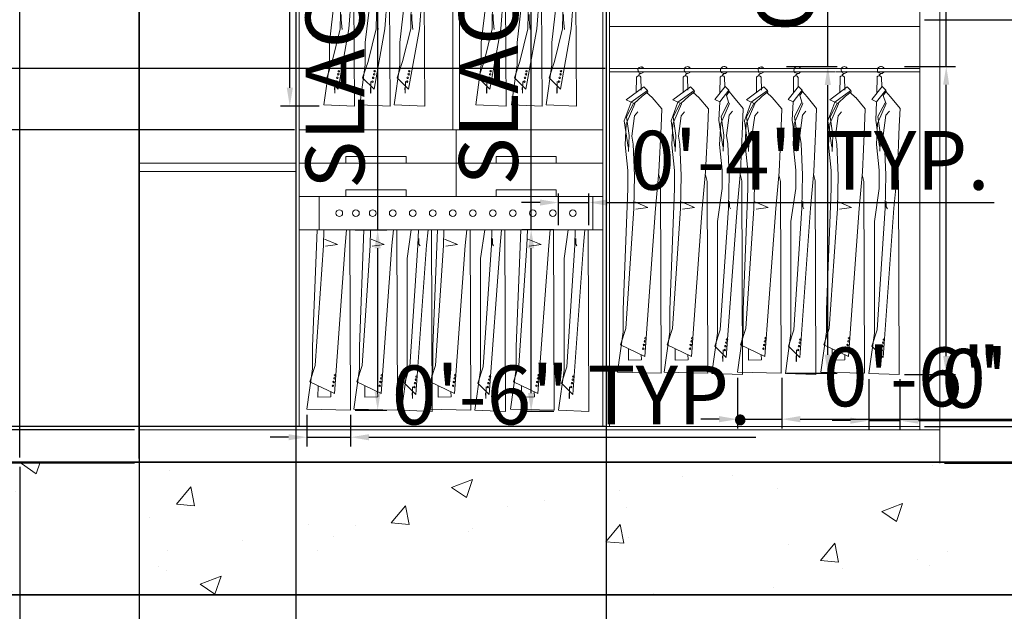
# Model space of a CAD drawing. Units: inches. Extents: x 2257 to 3678, y 834 to 1975.
# Tile 12 of 16: x 3338 to 3471, y 1677 to 1757. Entities that reach past the tile are written whole.
import ezdxf

# ---------------------------------------------------------------- set-up
doc = ezdxf.new("R2010")
doc.units = ezdxf.units.IN
for name, color, linetype, lineweight in [('A-ANNO-DIMS', 2, 'Continuous', 18), ('A-FURN-ELEV', 8, 'Continuous', 13), ('A-SECT', 7, 'Continuous', 35), ('A-SECT-CONC-PATT', 252, 'Continuous', 13)]:
    doc.layers.add(name, color=color, linetype=linetype, lineweight=lineweight)
doc.styles.get("Standard").update_dxf_attribs({"font": 'arial.ttf'})
doc.dimstyles.new('ISO-25', dxfattribs={"dimtxt": 8, "dimasz": 2.5, "dimexe": 1.25, "dimexo": 0.625, "dimtad": 1, "dimdec": 0, "dimlunit": 3, "dimtxsty": 'Standard', "dimcen": 2.5, "dimadec": 0, "dimazin": 0, "dimtfac": 1, "dimtdec": 0, "dimtmove": 0, "dimatfit": 3, "dimfxl": 1, "dimarcsym": 0})

# ---------------------------------------------------------------- blocks, each defined once
blk = doc.blocks.new('WARDROBE-JACKET-SHORT')
for p, q in [((1.8, 28.09), (0.39, 26.33)), ((1.11, 29.37), (1.09, 27.21)), ((1.75, 28.02), (1.71, 29.34)), ((1.8, 28.09), (2.29, 27.6)), ((1.06, 26.01), (2.29, 27.6)), ((2.34, 27.43), (1.96, 26.84)), ((2.29, 25.81), (1.96, 26.84)), ((2.34, 27.43), (2.29, 27.6)), ((2.33, 27.41), (2.93, 26.66)), ((0.39, 26.33), (1.06, 26.01)), ((1.06, 26.01), (0.94, 23.49)), ((2.36, 25.78), (1.19, 23.07)), ((1.23, 24.01), (2.2, 25.86)), ((2.94, 26.66), (4.23, 25.09)), ((1.96, 21.41), (2.32, 24.17)), ((2.32, 24.17), (2.79, 24.73)), ((4.23, 25.09), (4.14, 22.7)), ((0.94, 23.49), (1.46, 19.92)), ((1.19, 23.07), (1.04, 20.22)), ((1.23, 24.01), (1.59, 21.47)), ((1.59, 21.47), (1.5, 19.31)), ((2.14, 20.31), (1.96, 21.41)), ((4.14, 22.7), (3.87, 16.54)), ((1.04, 20.22), (1.4, 16.72)), ((2.32, 16.07), (2.14, 20.31)), ((1.4, 16.72), (1.4, 14.23)), ((2.23, 10.49), (2.32, 16.07)), ((3.87, 16.54), (3.41, 10.49)), ((4.05, 15.25), (3.83, 16.16)), ((4.14, 0), (4.05, 15.25)), ((1.4, 14.23), (0.76, 8.65)), ((2.37, 12.45), (2.37, 11.72)), ((2.37, 11.72), (2.51, 10.41)), ((1.13, 6.07), (2.23, 10.49)), ((3.41, 10.49), (1.94, 2.29)), ((0.76, 8.65), (0.76, 5.61)), ((0.76, 5.61), (0, 0.16)), ((0.4, 3.86), (1.13, 6.07)), ((1.94, 2.29), (0.4, 3.86)), ((1.51, 3.33), (1.49, 1.77)), ((1.47, 1.8), (1.45, 2.53)), ((1.49, 1.77), (1.47, 1.8)), ((0, 0.16), (4.14, 0))]:
    blk.add_line(p, q)
for centre, radius in [((1.45, 30.04), 0.0434), ((1.96, 4.32), 0.103), ((2.03, 4.74), 0.103), ((1.74, 3.32), 0.103), ((1.83, 3.84), 0.103)]:
    blk.add_circle(centre, radius)
for centre, radius, start, end in [((1.64, 30.31), 0.481, 28.9305, 230.329), ((1.4, 29.2), 0.341, 24.2419, 150.7783), ((1.75, 29.53), 0.361, 98.1438, 177.8717), ((1.75, 29.53), 0.315, 98.1438, 177.7449), ((1.64, 30.31), 0.481, 278.1438, 332.6972)]:
    blk.add_arc(centre, radius, start, end)
blk = doc.blocks.new('WARDROBE-JACKET-SHORT-B')
for p, q in [((1.11, 29.37), (1.09, 27.21)), ((1.75, 28.02), (1.72, 29.34)), ((1.8, 28.09), (2.29, 27.6)), ((1.06, 26.01), (2.29, 27.6)), ((2.34, 27.43), (1.96, 26.84)), ((2.29, 25.81), (1.96, 26.84)), ((2.34, 27.43), (2.29, 27.6)), ((2.33, 27.41), (2.94, 26.66)), ((1.06, 26.01), (0.94, 23.49)), ((2.36, 25.78), (1.19, 23.07)), ((1.23, 24.01), (2.2, 25.86)), ((2.94, 26.66), (4.23, 25.09)), ((1.96, 21.41), (2.33, 24.17)), ((2.33, 24.17), (2.79, 24.73)), ((4.23, 25.09), (4.14, 22.7)), ((0.94, 23.49), (1.46, 19.92)), ((1.19, 23.07), (1.04, 20.22)), ((1.23, 24.01), (1.59, 21.47)), ((1.59, 21.47), (1.5, 19.31)), ((2.14, 20.31), (1.96, 21.41)), ((4.14, 22.7), (3.87, 16.54)), ((1.04, 20.22), (1.4, 16.72)), ((2.33, 16.07), (2.14, 20.31)), ((1.4, 16.72), (1.4, 14.23)), ((2.23, 10.49), (2.33, 16.07)), ((3.87, 16.54), (3.41, 10.49)), ((4.05, 15.25), (3.83, 16.16)), ((4.14, 0), (4.05, 15.25)), ((1.4, 14.23), (0.76, 8.65)), ((2.37, 12.45), (2.37, 11.72)), ((2.37, 11.72), (2.52, 10.41)), ((1.13, 6.07), (2.23, 10.49)), ((3.41, 10.49), (1.94, 2.29)), ((0.76, 8.65), (0.76, 5.61)), ((0.76, 5.61), (0, 0.16)), ((0.4, 3.86), (1.13, 6.07)), ((1.94, 2.29), (0.4, 3.86)), ((1.51, 3.33), (1.49, 1.77)), ((1.47, 1.8), (1.45, 2.53)), ((1.49, 1.77), (1.47, 1.8)), ((0, 0.16), (4.14, 0))]:
    blk.add_line(p, q)
for centre, radius in [((1.45, 30.04), 0.0434), ((1.96, 4.32), 0.103), ((2.03, 4.74), 0.103), ((1.74, 3.32), 0.103), ((1.83, 3.84), 0.103)]:
    blk.add_circle(centre, radius)
for centre, radius, start, end in [((1.4, 29.2), 0.341, 24.2419, 150.7783), ((1.67, 30.37), 0.367, 58.8889, 230.4094), ((1.75, 29.53), 0.361, 98.1438, 177.8717), ((1.75, 29.53), 0.315, 98.1438, 177.7449), ((1.64, 30.31), 0.481, 278.1438, 332.6972), ((1.64, 30.31), 0.481, 28.9305, 58.8889)]:
    blk.add_arc(centre, radius, start, end)
blk = doc.blocks.new('WARDROBE-COAT')
for p, q in [((2.59, 40.24), (2.57, 38.08)), ((3.24, 38.47), (3.19, 40.21)), ((3.58, 38.9), (1.2, 37.14)), ((3.58, 38.9), (4.07, 38.41)), ((1.87, 36.82), (4.07, 38.41)), ((2.29, 36.62), (3.34, 37.65)), ((4.11, 38.23), (3.34, 37.65)), ((3.96, 38.12), (4.71, 37.47)), ((4.11, 38.23), (4.07, 38.41)), ((4.72, 37.47), (6.01, 35.9)), ((1.87, 36.82), (0.94, 34.3)), ((2.36, 36.59), (1.19, 33.88)), ((1.2, 37.14), (2.36, 36.59)), ((1.23, 34.82), (2.2, 36.66)), ((1.23, 34.82), (1.59, 32.28)), ((1.96, 32.22), (2.33, 34.98)), ((2.33, 34.98), (2.79, 35.53)), ((6.01, 35.9), (5.92, 33.51)), ((0.94, 34.3), (1.46, 30.72)), ((1.19, 33.88), (1.04, 31.02)), ((5.92, 33.51), (5.64, 27.34)), ((1.59, 32.28), (1.5, 30.12)), ((2.14, 31.12), (1.96, 32.22)), ((1.04, 31.02), (1.4, 27.53)), ((2.33, 26.88), (2.14, 31.12)), ((1.4, 27.53), (1.4, 25.04)), ((2.23, 22.37), (2.33, 26.88)), ((5.64, 27.34), (5.18, 22.37)), ((5.83, 26.06), (5.61, 26.97)), ((5.92, 0), (5.83, 26.06)), ((1.4, 25.04), (0.76, 8.65)), ((2.37, 23.26), (4.14, 22.52)), ((1.13, 6.07), (2.23, 22.37)), ((4.14, 22.52), (2.52, 22.29)), ((5.18, 22.37), (3.72, 2.29)), ((0.76, 8.65), (0.76, 5.61)), ((0.76, 5.61), (0, 0.16)), ((0.4, 3.86), (1.13, 6.07)), ((3.72, 2.29), (0.4, 3.86)), ((1.51, 3.33), (1.49, 1.77)), ((1.49, 1.77), (3.25, 1.8)), ((3.25, 1.8), (3.22, 2.53)), ((0, 0.16), (5.92, 0))]:
    blk.add_line(p, q)
for centre, radius in [((2.93, 40.91), 0.0434), ((3.74, 4.32), 0.103), ((3.81, 4.74), 0.103), ((3.52, 3.32), 0.103), ((3.61, 3.84), 0.103)]:
    blk.add_circle(centre, radius)
for centre, radius, start, end in [((3.15, 41.24), 0.367, 58.8889, 230.4094), ((3.12, 41.19), 0.481, 28.9305, 58.8889), ((2.88, 40.07), 0.341, 24.2419, 150.7783), ((3.23, 40.4), 0.361, 98.1438, 177.8717), ((3.23, 40.4), 0.315, 98.1438, 177.7449), ((3.12, 41.19), 0.481, 278.1438, 332.6972)]:
    blk.add_arc(centre, radius, start, end)
blk = doc.blocks.new('WARDROBE-COAT-B')
for p, q in [((2.59, 40.24), (2.57, 38.08)), ((3.24, 38.47), (3.19, 40.21)), ((3.58, 38.9), (1.2, 37.14)), ((3.58, 38.9), (4.07, 38.41)), ((1.87, 36.82), (4.07, 38.41)), ((2.29, 36.62), (3.34, 37.65)), ((4.11, 38.23), (3.34, 37.65)), ((3.96, 38.12), (4.71, 37.47)), ((4.11, 38.23), (4.07, 38.41)), ((4.72, 37.47), (6.01, 35.9)), ((1.87, 36.82), (0.94, 34.3)), ((2.36, 36.59), (1.19, 33.88)), ((1.2, 37.14), (2.36, 36.59)), ((1.23, 34.82), (2.2, 36.66)), ((1.23, 34.82), (1.59, 32.28)), ((1.96, 32.22), (2.33, 34.98)), ((2.33, 34.98), (2.79, 35.53)), ((6.01, 35.9), (5.92, 33.51)), ((0.94, 34.3), (1.46, 30.72)), ((1.19, 33.88), (1.04, 31.02)), ((5.92, 33.51), (5.64, 27.34)), ((1.59, 32.28), (1.5, 30.12)), ((2.14, 31.12), (1.96, 32.22)), ((1.04, 31.02), (1.4, 27.53)), ((2.33, 26.88), (2.14, 31.12)), ((1.4, 27.53), (1.4, 25.04)), ((2.23, 22.37), (2.33, 26.88)), ((5.64, 27.34), (5.18, 22.37)), ((5.83, 26.06), (5.61, 26.97)), ((5.92, 0), (5.83, 26.06)), ((1.4, 25.04), (0.76, 8.65)), ((2.37, 23.26), (4.14, 22.52)), ((1.13, 6.07), (2.23, 22.37)), ((4.14, 22.52), (2.52, 22.29)), ((5.18, 22.37), (3.72, 2.29)), ((0.76, 8.65), (0.76, 5.61)), ((0.76, 5.61), (0, 0.16)), ((0.4, 3.86), (1.13, 6.07)), ((3.72, 2.29), (0.4, 3.86)), ((1.51, 3.33), (1.49, 1.77)), ((1.49, 1.77), (3.25, 1.8)), ((3.25, 1.8), (3.22, 2.53)), ((0, 0.16), (5.92, 0))]:
    blk.add_line(p, q)
for centre, radius in [((2.93, 40.91), 0.0434), ((3.74, 4.32), 0.103), ((3.81, 4.74), 0.103), ((3.52, 3.32), 0.103), ((3.61, 3.84), 0.103)]:
    blk.add_circle(centre, radius)
for centre, radius, start, end in [((3.15, 41.24), 0.412, 58.8889, 230.4094), ((3.12, 41.19), 0.481, 28.9305, 58.8889), ((2.88, 40.07), 0.341, 24.2419, 150.7783), ((3.23, 40.4), 0.361, 98.1438, 177.8717), ((3.23, 40.4), 0.315, 98.1438, 177.7449), ((3.12, 41.19), 0.481, 278.1438, 332.6972)]:
    blk.add_arc(centre, radius, start, end)
blk = doc.blocks.new('WARDROBE-JACKET-LONG')
for p, q in [((1.11, 40.4), (1.09, 38.25)), ((1.75, 39.06), (1.72, 40.38)), ((1.8, 39.13), (0.39, 37.37)), ((1.8, 39.13), (2.29, 38.64)), ((1.06, 37.05), (2.29, 38.64)), ((2.34, 38.46), (1.96, 37.88)), ((2.29, 36.85), (1.96, 37.88)), ((2.34, 38.46), (2.29, 38.64)), ((2.33, 38.45), (2.94, 37.7)), ((2.94, 37.7), (4.24, 36.13)), ((0.39, 37.37), (1.06, 37.05)), ((1.06, 37.05), (0.94, 34.53)), ((2.36, 36.82), (1.19, 34.11)), ((1.23, 35.05), (2.2, 36.89)), ((4.24, 36.13), (4.14, 33.74)), ((1.23, 35.05), (1.59, 32.51)), ((1.96, 32.45), (2.33, 35.21)), ((2.33, 35.21), (2.79, 35.76)), ((0.94, 34.53), (1.46, 30.95)), ((1.19, 34.11), (1.04, 31.25)), ((4.14, 33.74), (3.87, 27.57)), ((1.59, 32.51), (1.5, 30.35)), ((2.14, 31.35), (1.96, 32.45)), ((1.04, 31.25), (1.4, 27.76)), ((2.33, 27.11), (2.14, 31.35)), ((1.4, 27.76), (1.4, 25.27)), ((2.23, 22.6), (2.33, 27.11)), ((3.87, 27.57), (3.41, 22.6)), ((4.05, 26.29), (3.83, 27.2)), ((4.14, 0), (4.05, 26.29)), ((1.4, 25.27), (0.76, 20.76)), ((2.37, 23.49), (2.37, 22.75)), ((2.37, 22.75), (2.52, 22.52)), ((1.13, 6.07), (2.23, 22.6)), ((3.41, 22.6), (1.94, 2.29)), ((0.76, 20.76), (0.76, 5.61)), ((0.76, 5.61), (0, 0.15)), ((0.4, 3.86), (1.13, 6.07)), ((1.94, 2.29), (0.4, 3.86)), ((1.51, 3.33), (1.49, 1.77)), ((1.47, 1.8), (1.45, 2.52)), ((1.49, 1.77), (1.47, 1.8)), ((0, 0.15), (4.14, 0))]:
    blk.add_line(p, q)
for centre, radius in [((1.45, 41.08), 0.0434), ((1.96, 4.32), 0.103), ((2.03, 4.74), 0.103), ((1.74, 3.32), 0.103), ((1.83, 3.84), 0.103)]:
    blk.add_circle(centre, radius)
for centre, radius, start, end in [((1.64, 41.35), 0.481, 28.9305, 230.329), ((1.4, 40.24), 0.341, 24.2419, 150.7783), ((1.75, 40.56), 0.361, 98.1438, 177.8717), ((1.75, 40.56), 0.315, 98.1438, 177.7449), ((1.64, 41.35), 0.481, 278.1438, 332.6972)]:
    blk.add_arc(centre, radius, start, end)
blk = doc.blocks.new('WARDROBE-GARMENT-LOWER')
for p, q in [((1.38, 24.51), (0.76, 8.65)), ((2.23, 22.37), (2.28, 24.51)), ((5.38, 24.51), (5.18, 22.37)), ((5.92, 0), (5.83, 24.51)), ((2.37, 23.26), (4.14, 22.52)), ((1.13, 6.07), (2.23, 22.37)), ((4.14, 22.52), (2.52, 22.29)), ((5.18, 22.37), (3.72, 2.29)), ((0.76, 8.65), (0.76, 5.61)), ((0.76, 5.61), (0, 0.16)), ((0.4, 3.86), (1.13, 6.07)), ((3.72, 2.29), (0.4, 3.86)), ((1.51, 3.33), (1.49, 1.77)), ((1.49, 1.77), (3.25, 1.8)), ((3.25, 1.8), (3.22, 2.52)), ((0, 0.16), (5.92, 0))]:
    blk.add_line(p, q)
for centre in [(3.74, 4.32), (3.81, 4.74), (3.52, 3.32), (3.61, 3.84)]:
    blk.add_circle(centre, 0.103)
blk = doc.blocks.new('WARDROBE-GARMENT-LOWER-B')
for p, q in [((1.32, 24.68), (0.76, 20.76)), ((2.23, 22.6), (2.28, 24.68)), ((3.6, 24.68), (3.41, 22.6)), ((4.14, 0), (4.06, 24.68)), ((2.37, 23.49), (2.37, 22.75)), ((2.37, 22.75), (2.51, 22.52)), ((1.13, 6.07), (2.23, 22.6)), ((3.41, 22.6), (1.94, 2.29)), ((0.76, 20.76), (0.76, 5.61)), ((0.76, 5.61), (0, 0.16)), ((0.4, 3.86), (1.13, 6.07)), ((1.94, 2.29), (0.4, 3.86)), ((1.51, 3.33), (1.49, 1.77)), ((1.47, 1.8), (1.45, 2.53)), ((1.49, 1.77), (1.47, 1.8)), ((0, 0.16), (4.14, 0))]:
    blk.add_line(p, q)
for centre in [(1.96, 4.32), (2.03, 4.74), (1.74, 3.32), (1.83, 3.84)]:
    blk.add_circle(centre, 0.103)
blk = doc.blocks.new('*D86')
at = {"layer": 'A-ANNO-DIMS', "color": 0, "lineweight": -2, "transparency": 16777216}
for p, q in [((3374.38, 1776.04), (3374.38, 1916.69)), ((3378.38, 1776.04), (3373.13, 1776.04)), ((3374.38, 1747.73), (3374.38, 1773.54)), ((3378.38, 1745.23), (3373.13, 1745.23))]:
    blk.add_line(p, q, dxfattribs=at)
at = {"layer": 'A-ANNO-DIMS', "color": 0, "transparency": 16777216}
for points in [[(3373.96, 1773.54), (3374.8, 1773.54), (3374.38, 1776.04)], [(3373.96, 1747.73), (3374.8, 1747.73), (3374.38, 1745.23)]]:
    blk.add_solid(points, dxfattribs=at)
at = {"layer": 'Defpoints', "color": 0, "transparency": 16777216}
for p in [(3374.38, 1776.04), (3379, 1776.04), (3379, 1745.23)]:
    blk.add_point(p, dxfattribs=at)
at = {"layer": 'A-ANNO-DIMS', "color": 0, "transparency": 16777216, "insert": (3369.62, 1847.62), "char_height": 8, "attachment_point": 5, "rotation": 90}
blk.add_mtext('SHORT JACKET 2\'-7" TYP.', dxfattribs=at)
blk = doc.blocks.new('*D88')
at = {"layer": 'A-ANNO-DIMS', "color": 0, "lineweight": -2, "transparency": 16777216}
for p, q in [((3386.31, 1728.42), (3386.31, 1846.75)), ((3383.26, 1728.42), (3387.56, 1728.42)), ((3386.31, 1706.41), (3386.31, 1725.92)), ((3383.26, 1703.91), (3387.56, 1703.91))]:
    blk.add_line(p, q, dxfattribs=at)
at = {"layer": 'A-ANNO-DIMS', "color": 0, "transparency": 16777216}
for points in [[(3385.89, 1725.92), (3386.72, 1725.92), (3386.31, 1728.42)], [(3385.89, 1706.41), (3386.72, 1706.41), (3386.31, 1703.91)]]:
    blk.add_solid(points, dxfattribs=at)
at = {"layer": 'Defpoints', "color": 0, "transparency": 16777216}
for p in [(3382.63, 1728.42), (3386.31, 1728.42), (3382.63, 1703.91)]:
    blk.add_point(p, dxfattribs=at)
at = {"layer": 'A-ANNO-DIMS', "color": 0, "transparency": 16777216, "insert": (3381.55, 1788.84), "char_height": 8, "attachment_point": 5, "rotation": 90}
blk.add_mtext('SLACKS 2\'-0 1/2" TYP.', dxfattribs=at)
blk = doc.blocks.new('*D89')
at = {"layer": 'A-ANNO-DIMS', "color": 0, "lineweight": -2, "transparency": 16777216}
for p, q in [((3376.71, 1703.29), (3376.71, 1698.99)), ((3382.63, 1703.29), (3382.63, 1698.99)), ((3374.21, 1700.24), (3371.71, 1700.24)), ((3376.71, 1700.24), (3382.63, 1700.24)), ((3385.13, 1700.24), (3437.65, 1700.24))]:
    blk.add_line(p, q, dxfattribs=at)
at = {"layer": 'A-ANNO-DIMS', "color": 0, "transparency": 16777216}
for points in [[(3374.21, 1700.65), (3374.21, 1699.82), (3376.71, 1700.24)], [(3385.13, 1700.65), (3385.13, 1699.82), (3382.63, 1700.24)]]:
    blk.add_solid(points, dxfattribs=at)
at = {"layer": 'Defpoints', "color": 0, "transparency": 16777216}
for p in [(3376.71, 1703.91), (3382.63, 1703.91), (3382.63, 1700.24)]:
    blk.add_point(p, dxfattribs=at)
at = {"layer": 'A-ANNO-DIMS', "color": 0, "transparency": 16777216, "insert": (3412.64, 1704.94), "char_height": 8, "attachment_point": 5}
blk.add_mtext('0\'-6" TYP.', dxfattribs=at)
blk = doc.blocks.new('*D90')
at = {"layer": 'A-ANNO-DIMS', "color": 0, "lineweight": -2, "transparency": 16777216}
for p, q in [((3463.51, 1750.62), (3463.51, 1883.51)), ((3457.86, 1750.62), (3464.76, 1750.62)), ((3463.51, 1711.27), (3463.51, 1748.12)), ((3457.86, 1708.77), (3464.76, 1708.77))]:
    blk.add_line(p, q, dxfattribs=at)
at = {"layer": 'A-ANNO-DIMS', "color": 0, "transparency": 16777216}
for points in [[(3463.09, 1748.12), (3463.92, 1748.12), (3463.51, 1750.62)], [(3463.09, 1711.27), (3463.92, 1711.27), (3463.51, 1708.77)]]:
    blk.add_solid(points, dxfattribs=at)
at = {"layer": 'Defpoints', "color": 0, "transparency": 16777216}
for p in [(3457.23, 1750.62), (3463.51, 1750.62), (3457.23, 1708.77)]:
    blk.add_point(p, dxfattribs=at)
at = {"layer": 'A-ANNO-DIMS', "color": 0, "transparency": 16777216, "insert": (3458.74, 1818.32), "char_height": 8, "attachment_point": 5, "rotation": 90}
blk.add_mtext('LONG JACKET 3\'-6" TYP.', dxfattribs=at)
blk = doc.blocks.new('*D91')
at = {"layer": 'A-ANNO-DIMS', "color": 0, "lineweight": -2, "transparency": 16777216}
for p, q in [((3453, 1708.14), (3453, 1701.24)), ((3457.23, 1708.14), (3457.23, 1701.24)), ((3450.5, 1702.49), (3448, 1702.49)), ((3453, 1702.49), (3457.23, 1702.49)), ((3459.73, 1702.49), (3512.24, 1702.49))]:
    blk.add_line(p, q, dxfattribs=at)
at = {"layer": 'A-ANNO-DIMS', "color": 0, "transparency": 16777216}
for points in [[(3450.5, 1702.91), (3450.5, 1702.08), (3453, 1702.49)], [(3459.73, 1702.91), (3459.73, 1702.08), (3457.23, 1702.49)]]:
    blk.add_solid(points, dxfattribs=at)
at = {"layer": 'Defpoints', "color": 0, "transparency": 16777216}
for p in [(3453, 1708.77), (3457.23, 1708.77), (3457.23, 1702.49)]:
    blk.add_point(p, dxfattribs=at)
at = {"layer": 'A-ANNO-DIMS', "color": 0, "transparency": 16777216, "insert": (3487.24, 1707.2), "char_height": 8, "attachment_point": 5}
blk.add_mtext('0\'-4" TYP.', dxfattribs=at)
blk = doc.blocks.new('*D92')
at = {"layer": 'A-ANNO-DIMS', "color": 0, "lineweight": -2, "transparency": 16777216}
for p, q in [((3447.43, 1750.59), (3447.43, 1855.81)), ((3441.81, 1750.59), (3448.68, 1750.59)), ((3447.43, 1711.44), (3447.43, 1748.09)), ((3441.81, 1708.94), (3448.68, 1708.94))]:
    blk.add_line(p, q, dxfattribs=at)
at = {"layer": 'A-ANNO-DIMS', "color": 0, "transparency": 16777216}
for points in [[(3447.01, 1748.09), (3447.85, 1748.09), (3447.43, 1750.59)], [(3447.01, 1711.44), (3447.85, 1711.44), (3447.43, 1708.94)]]:
    blk.add_solid(points, dxfattribs=at)
at = {"layer": 'Defpoints', "color": 0, "transparency": 16777216}
for p in [(3441.18, 1750.59), (3447.43, 1750.59), (3441.18, 1708.94)]:
    blk.add_point(p, dxfattribs=at)
at = {"layer": 'A-ANNO-DIMS', "color": 0, "transparency": 16777216, "insert": (3442.66, 1804.45), "char_height": 8, "attachment_point": 5, "rotation": 90}
blk.add_mtext('COAT 3\'-5 1/2" TYP.', dxfattribs=at)
blk = doc.blocks.new('*D93')
at = {"layer": 'A-ANNO-DIMS', "color": 0, "lineweight": -2, "transparency": 16777216}
for p, q in [((3435.17, 1708.31), (3435.17, 1701.44)), ((3441.18, 1708.31), (3441.18, 1701.44)), ((3432.67, 1702.69), (3430.17, 1702.69)), ((3435.17, 1702.69), (3441.18, 1702.69)), ((3443.68, 1702.69), (3496.2, 1702.69))]:
    blk.add_line(p, q, dxfattribs=at)
at = {"layer": 'A-ANNO-DIMS', "color": 0, "transparency": 16777216}
for points in [[(3432.67, 1703.11), (3432.67, 1702.27), (3435.17, 1702.69)], [(3443.68, 1703.11), (3443.68, 1702.27), (3441.18, 1702.69)]]:
    blk.add_solid(points, dxfattribs=at)
at = {"layer": 'Defpoints', "color": 0, "transparency": 16777216}
for p in [(3435.17, 1708.94), (3441.18, 1708.94), (3441.18, 1702.69)]:
    blk.add_point(p, dxfattribs=at)
at = {"layer": 'A-ANNO-DIMS', "color": 0, "transparency": 16777216, "insert": (3471.19, 1707.4), "char_height": 8, "attachment_point": 5}
blk.add_mtext('0\'-6" TYP.', dxfattribs=at)
blk = doc.blocks.new('*D94')
at = {"layer": 'A-ANNO-DIMS', "color": 0, "lineweight": -2, "transparency": 16777216}
for p, q in [((3407.15, 1728.42), (3407.15, 1857.31)), ((3410.23, 1728.42), (3405.9, 1728.42)), ((3407.15, 1706.24), (3407.15, 1725.92)), ((3410.23, 1703.74), (3405.9, 1703.74))]:
    blk.add_line(p, q, dxfattribs=at)
at = {"layer": 'A-ANNO-DIMS', "color": 0, "transparency": 16777216}
for points in [[(3406.73, 1725.92), (3407.57, 1725.92), (3407.15, 1728.42)], [(3406.73, 1706.24), (3407.57, 1706.24), (3407.15, 1703.74)]]:
    blk.add_solid(points, dxfattribs=at)
at = {"layer": 'Defpoints', "color": 0, "transparency": 16777216}
for p in [(3407.15, 1728.42), (3410.85, 1728.42), (3410.85, 1703.74)]:
    blk.add_point(p, dxfattribs=at)
at = {"layer": 'A-ANNO-DIMS', "color": 0, "transparency": 16777216, "insert": (3402.39, 1794.12), "char_height": 8, "attachment_point": 5, "rotation": 90}
blk.add_mtext('SLACKS B 2\'-0 1/2" TYP.', dxfattribs=at)
blk = doc.blocks.new('*D95')
at = {"layer": 'A-ANNO-DIMS', "color": 0, "lineweight": -2, "transparency": 16777216}
for p, q in [((3410.85, 1729.05), (3410.85, 1733.37)), ((3414.99, 1729.05), (3414.99, 1733.37)), ((3408.35, 1732.12), (3405.85, 1732.12)), ((3410.85, 1732.12), (3414.99, 1732.12)), ((3417.49, 1732.12), (3470.01, 1732.12))]:
    blk.add_line(p, q, dxfattribs=at)
at = {"layer": 'A-ANNO-DIMS', "color": 0, "transparency": 16777216}
for points in [[(3408.35, 1732.54), (3408.35, 1731.71), (3410.85, 1732.12)], [(3417.49, 1732.54), (3417.49, 1731.71), (3414.99, 1732.12)]]:
    blk.add_solid(points, dxfattribs=at)
at = {"layer": 'Defpoints', "color": 0, "transparency": 16777216}
for p in [(3414.99, 1732.12), (3410.85, 1728.42), (3414.99, 1728.42)]:
    blk.add_point(p, dxfattribs=at)
at = {"layer": 'A-ANNO-DIMS', "color": 0, "transparency": 16777216, "insert": (3445, 1736.83), "char_height": 8, "attachment_point": 5}
blk.add_mtext('0\'-4" TYP.', dxfattribs=at)
blk = doc.blocks.new('*D137')
at = {"layer": 'A-ANNO-DIMS', "color": 0, "lineweight": -2, "transparency": 16777216}
for p, q in [((3337.7, 1696.22), (3337.7, 1600.44)), ((3493.7, 1696.22), (3493.7, 1600.44)), ((3340.2, 1601.69), (3491.2, 1601.69))]:
    blk.add_line(p, q, dxfattribs=at)
at = {"layer": 'A-ANNO-DIMS', "color": 0, "transparency": 16777216}
for points in [[(3340.2, 1602.1), (3340.2, 1601.27), (3337.7, 1601.69)], [(3491.2, 1602.1), (3491.2, 1601.27), (3493.7, 1601.69)]]:
    blk.add_solid(points, dxfattribs=at)
at = {"layer": 'Defpoints', "color": 0, "transparency": 16777216}
for p in [(3337.7, 1696.84), (3493.7, 1696.84), (3493.7, 1601.69)]:
    blk.add_point(p, dxfattribs=at)
at = {"layer": 'A-ANNO-DIMS', "color": 0, "transparency": 16777216, "insert": (3415.7, 1606.4), "char_height": 8, "attachment_point": 5}
blk.add_mtext('13\'-0"', dxfattribs=at)
blk = doc.blocks.new('*D139')
at = {"layer": 'A-ANNO-DIMS', "color": 0, "lineweight": -2, "transparency": 16777216}
for p, q in [((3463.29, 1805.46), (3573.28, 1805.46)), ((3572.03, 1699.2), (3572.03, 1802.96)), ((3463.29, 1696.7), (3573.28, 1696.7))]:
    blk.add_line(p, q, dxfattribs=at)
at = {"layer": 'A-ANNO-DIMS', "color": 0, "transparency": 16777216}
for points in [[(3571.61, 1802.96), (3572.45, 1802.96), (3572.03, 1805.46)], [(3571.61, 1699.2), (3572.45, 1699.2), (3572.03, 1696.7)]]:
    blk.add_solid(points, dxfattribs=at)
at = {"layer": 'Defpoints', "color": 0, "transparency": 16777216}
for p in [(3462.66, 1805.46), (3572.03, 1805.46), (3462.66, 1696.7)]:
    blk.add_point(p, dxfattribs=at)
at = {"layer": 'A-ANNO-DIMS', "color": 0, "transparency": 16777216, "insert": (3567.32, 1751.08), "char_height": 8, "attachment_point": 5, "rotation": 90}
blk.add_mtext('9\'-1"', dxfattribs=at)
blk = doc.blocks.new('*D140')
at = {"layer": 'A-ANNO-DIMS', "color": 0, "lineweight": -2, "transparency": 16777216}
for p, q in [((3337.7, 1697.47), (3337.7, 1897.74)), ((3353.91, 1697.33), (3353.91, 1897.74)), ((3340.2, 1896.49), (3351.41, 1896.49)), ((3353.91, 1896.49), (3378.17, 1896.49))]:
    blk.add_line(p, q, dxfattribs=at)
at = {"layer": 'A-ANNO-DIMS', "color": 0, "transparency": 16777216}
for points in [[(3340.2, 1896.91), (3340.2, 1896.07), (3337.7, 1896.49)], [(3351.41, 1896.91), (3351.41, 1896.07), (3353.91, 1896.49)]]:
    blk.add_solid(points, dxfattribs=at)
at = {"layer": 'Defpoints', "color": 0, "transparency": 16777216}
for p in [(3353.91, 1896.49), (3337.7, 1696.84), (3353.91, 1696.7)]:
    blk.add_point(p, dxfattribs=at)
at = {"layer": 'A-ANNO-DIMS', "color": 0, "transparency": 16777216, "insert": (3367.29, 1901.13), "char_height": 8, "attachment_point": 5}
blk.add_mtext('1\'-4"', dxfattribs=at)
blk = doc.blocks.new('*D143')
at = {"layer": 'A-ANNO-DIMS', "color": 0, "lineweight": -2, "transparency": 16777216}
for p, q in [((3353.91, 1804.83), (3353.91, 1600.44)), ((3375.21, 1803.92), (3375.21, 1600.44)), ((3356.41, 1601.69), (3372.71, 1601.69)), ((3375.21, 1601.69), (3418.11, 1601.69))]:
    blk.add_line(p, q, dxfattribs=at)
at = {"layer": 'A-ANNO-DIMS', "color": 0, "transparency": 16777216}
for points in [[(3356.41, 1602.1), (3356.41, 1601.27), (3353.91, 1601.69)], [(3372.71, 1602.1), (3372.71, 1601.27), (3375.21, 1601.69)]]:
    blk.add_solid(points, dxfattribs=at)
at = {"layer": 'Defpoints', "color": 0, "transparency": 16777216}
for p in [(3353.91, 1805.46), (3375.21, 1804.55), (3375.21, 1601.69)]:
    blk.add_point(p, dxfattribs=at)
at = {"layer": 'A-ANNO-DIMS', "color": 0, "transparency": 16777216, "insert": (3397.91, 1606.45), "char_height": 8, "attachment_point": 5}
blk.add_mtext('1\'-9 1/2"', dxfattribs=at)
blk = doc.blocks.new('*D144')
at = {"layer": 'A-ANNO-DIMS', "color": 0, "lineweight": -2, "transparency": 16777216}
for p, q in [((3375.21, 1803.92), (3375.21, 1600.44)), ((3417.35, 1803.92), (3417.35, 1600.44)), ((3377.71, 1601.69), (3414.85, 1601.69))]:
    blk.add_line(p, q, dxfattribs=at)
at = {"layer": 'A-ANNO-DIMS', "color": 0, "transparency": 16777216}
for points in [[(3377.71, 1602.1), (3377.71, 1601.27), (3375.21, 1601.69)], [(3414.85, 1602.1), (3414.85, 1601.27), (3417.35, 1601.69)]]:
    blk.add_solid(points, dxfattribs=at)
at = {"layer": 'Defpoints', "color": 0, "transparency": 16777216}
for p in [(3375.21, 1804.55), (3417.35, 1804.55), (3417.35, 1601.69)]:
    blk.add_point(p, dxfattribs=at)
at = {"layer": 'A-ANNO-DIMS', "color": 0, "transparency": 16777216, "insert": (3396.28, 1606.4), "char_height": 8, "attachment_point": 5}
blk.add_mtext('3\'-6"', dxfattribs=at)
blk = doc.blocks.new('*D146')
at = {"layer": 'A-ANNO-DIMS', "color": 0, "lineweight": -2, "transparency": 16777216}
for p, q in [((2973.05, 1703.73), (2973.05, 1747.39)), ((3353.28, 1701.23), (2971.8, 1701.23)), ((2973.05, 1696.7), (2973.05, 1701.23)), ((3353.28, 1696.7), (2971.8, 1696.7)), ((2973.05, 1694.2), (2973.05, 1691.7))]:
    blk.add_line(p, q, dxfattribs=at)
at = {"layer": 'A-ANNO-DIMS', "color": 0, "transparency": 16777216}
for points in [[(2972.63, 1703.73), (2973.47, 1703.73), (2973.05, 1701.23)], [(2972.63, 1694.2), (2973.47, 1694.2), (2973.05, 1696.7)]]:
    blk.add_solid(points, dxfattribs=at)
at = {"layer": 'Defpoints', "color": 0, "transparency": 16777216}
for p in [(2973.05, 1701.23), (3353.91, 1701.23), (3353.91, 1696.7)]:
    blk.add_point(p, dxfattribs=at)
at = {"layer": 'A-ANNO-DIMS', "color": 0, "transparency": 16777216, "insert": (2968.29, 1726.81), "char_height": 8, "attachment_point": 5, "rotation": 90}
blk.add_mtext('0\'-4 1/2"', dxfattribs=at)
blk = doc.blocks.new('*D147')
at = {"layer": 'A-ANNO-DIMS', "color": 0, "lineweight": -2, "transparency": 16777216}
for p, q in [((3460.57, 1756.97), (3573.28, 1756.97)), ((3572.03, 1704.19), (3572.03, 1754.47)), ((3460.57, 1701.69), (3573.28, 1701.69))]:
    blk.add_line(p, q, dxfattribs=at)
at = {"layer": 'A-ANNO-DIMS', "color": 0, "transparency": 16777216}
for points in [[(3571.61, 1754.47), (3572.45, 1754.47), (3572.03, 1756.97)], [(3571.61, 1704.19), (3572.45, 1704.19), (3572.03, 1701.69)]]:
    blk.add_solid(points, dxfattribs=at)
at = {"layer": 'Defpoints', "color": 0, "transparency": 16777216}
for p in [(3459.94, 1756.97), (3572.03, 1756.97), (3459.94, 1701.69)]:
    blk.add_point(p, dxfattribs=at)
at = {"layer": 'A-ANNO-DIMS', "color": 0, "transparency": 16777216, "insert": (3567.27, 1729.33), "char_height": 8, "attachment_point": 5, "rotation": 90}
blk.add_mtext('4\'-7 1/2"', dxfattribs=at)
blk = doc.blocks.new('*D148')
at = {"layer": 'A-ANNO-DIMS', "color": 0, "lineweight": -2, "transparency": 16777216}
for p, q in [((3375.03, 1775.78), (2971.8, 1775.78)), ((2973.05, 1744.52), (2973.05, 1773.28)), ((3375.03, 1742.02), (2971.8, 1742.02))]:
    blk.add_line(p, q, dxfattribs=at)
at = {"layer": 'A-ANNO-DIMS', "color": 0, "transparency": 16777216}
for points in [[(2972.63, 1773.28), (2973.47, 1773.28), (2973.05, 1775.78)], [(2972.63, 1744.52), (2973.47, 1744.52), (2973.05, 1742.02)]]:
    blk.add_solid(points, dxfattribs=at)
at = {"layer": 'Defpoints', "color": 0, "transparency": 16777216}
for p in [(2973.05, 1775.78), (3375.66, 1775.78), (3375.66, 1742.02)]:
    blk.add_point(p, dxfattribs=at)
at = {"layer": 'A-ANNO-DIMS', "color": 0, "transparency": 16777216, "insert": (2968.34, 1758.9), "char_height": 8, "attachment_point": 5, "rotation": 90}
blk.add_mtext('2\'-10"', dxfattribs=at)
blk = doc.blocks.new('*D149')
at = {"layer": 'A-ANNO-DIMS', "color": 0, "lineweight": -2, "transparency": 16777216}
for p, q in [((3417.18, 1750.35), (2971.8, 1750.35)), ((2973.05, 1704.19), (2973.05, 1747.85)), ((3417.18, 1701.69), (2971.8, 1701.69))]:
    blk.add_line(p, q, dxfattribs=at)
at = {"layer": 'A-ANNO-DIMS', "color": 0, "transparency": 16777216}
for points in [[(2972.63, 1747.85), (2973.47, 1747.85), (2973.05, 1750.35)], [(2972.63, 1704.19), (2973.47, 1704.19), (2973.05, 1701.69)]]:
    blk.add_solid(points, dxfattribs=at)
at = {"layer": 'Defpoints', "color": 0, "transparency": 16777216}
for p in [(2973.05, 1750.35), (3417.8, 1750.35), (3417.8, 1701.69)]:
    blk.add_point(p, dxfattribs=at)
at = {"layer": 'A-ANNO-DIMS', "color": 0, "transparency": 16777216, "insert": (2968.29, 1726.02), "char_height": 8, "attachment_point": 5, "rotation": 90}
blk.add_mtext('4\'-0 1/2"', dxfattribs=at)

msp = doc.modelspace()

# ---------------------------------------------------------------- hatches: boundary and pattern name
at = {"layer": 'A-SECT-CONC-PATT'}
h = msp.add_hatch(dxfattribs=at)
h.set_pattern_fill('AR-CONC', color=256, scale=0.16, style=0)
h.paths.add_polyline_path([(3004.7, 1678.84), (3502.7, 1678.84), (3502.7, 1696.84), (3004.7, 1696.84)])

# ---------------------------------------------------------------- linework, layer by layer
at = {"layer": 'A-FURN-ELEV'}
for p, q in [((3353.91, 1696.7), (3353.91, 1805.46)), ((3462.66, 1696.7), (3462.66, 1805.46)), ((3459.94, 1701.23), (3459.94, 1804.55)), ((3375.21, 1701.69), (3375.21, 1778.72)), ((3375.66, 1701.69), (3375.66, 1778.72)), ((3396.5, 1742.02), (3396.5, 1778.72)), ((3397.41, 1742.02), (3397.41, 1778.72)), ((3416.89, 1701.69), (3416.89, 1778.72)), ((3417.8, 1701.69), (3417.8, 1778.72)), ((3417.8, 1756.06), (3459.94, 1756.06)), ((3417.8, 1750.35), (3459.94, 1750.35)), ((3417.8, 1749.9), (3448.44, 1749.9)), ((3448.51, 1749.9), (3459.94, 1749.9)), ((3375.66, 1742.02), (3416.89, 1742.02)), ((3396.96, 1742.02), (3396.96, 1732.95)), ((3375.21, 1737.49), (3353.91, 1737.49)), ((3375.66, 1737.49), (3416.89, 1737.49)), ((3375.21, 1736.35), (3353.91, 1736.35)), ((3375.66, 1732.95), (3416.89, 1732.95)), ((3378.38, 1732.95), (3378.38, 1728.42)), ((3415.54, 1732.95), (3415.54, 1728.42)), ((3375.66, 1728.42), (3416.89, 1728.42)), ((3459.94, 1701.69), (3353.91, 1701.69)), ((3462.66, 1701.23), (3353.91, 1701.23))]:
    msp.add_line(p, q, dxfattribs=at)
for points in [[(3390.16, 1737.49), (3390.16, 1738.39), (3382, 1738.39), (3382, 1737.49)], [(3410.55, 1737.49), (3410.55, 1738.39), (3402.39, 1738.39), (3402.39, 1737.49)], [(3390.16, 1732.95), (3390.16, 1733.86), (3382, 1733.86), (3382, 1732.95)], [(3410.55, 1732.95), (3410.55, 1733.86), (3402.39, 1733.86), (3402.39, 1732.95)]]:
    msp.add_lwpolyline(points, dxfattribs=at)
for centre in [(3381.1, 1730.69), (3383.36, 1730.69), (3385.63, 1730.69), (3388.35, 1730.69), (3391.07, 1730.69), (3393.78, 1730.69), (3396.5, 1730.69), (3399.22, 1730.69), (3401.94, 1730.69), (3404.66, 1730.69), (3407.38, 1730.69), (3410.1, 1730.69), (3412.82, 1730.69)]:
    msp.add_circle(centre, 0.453, dxfattribs=at)
at = {"layer": 'A-SECT'}
for p, q in [((3502.7, 1696.84), (3004.7, 1696.84)), ((3502.7, 1678.84), (3004.7, 1678.84))]:
    msp.add_line(p, q, dxfattribs=at)

# ---------------------------------------------------------------- block references
at = {"layer": 'A-FURN-ELEV'}
for name, p in [('WARDROBE-JACKET-SHORT', (3379, 1745.23)), ('WARDROBE-JACKET-SHORT-B', (3383.87, 1745.23)), ('WARDROBE-JACKET-SHORT', (3388.56, 1745.23)), ('WARDROBE-JACKET-SHORT', (3399.62, 1745.23)), ('WARDROBE-JACKET-SHORT-B', (3404.49, 1745.23)), ('WARDROBE-JACKET-SHORT', (3409.18, 1745.23)), ('WARDROBE-COAT', (3418.86, 1708.94)), ('WARDROBE-COAT-B', (3425.2, 1708.94)), ('WARDROBE-JACKET-LONG', (3431.7, 1708.77)), ('WARDROBE-COAT', (3435.17, 1708.94)), ('WARDROBE-JACKET-LONG', (3441.67, 1708.77)), ('WARDROBE-COAT-B', (3446.5, 1708.94)), ('WARDROBE-JACKET-LONG', (3453, 1708.77)), ('WARDROBE-GARMENT-LOWER', (3376.71, 1703.91)), ('WARDROBE-GARMENT-LOWER', (3383.06, 1703.91)), ('WARDROBE-GARMENT-LOWER-B', (3389.55, 1703.74)), ('WARDROBE-GARMENT-LOWER', (3393.03, 1703.91)), ('WARDROBE-GARMENT-LOWER-B', (3399.52, 1703.74)), ('WARDROBE-GARMENT-LOWER', (3404.35, 1703.91)), ('WARDROBE-GARMENT-LOWER-B', (3410.85, 1703.74))]:
    msp.add_blockref(name, p, dxfattribs=at)

# ---------------------------------------------------------------- dimensions: what is measured, and where the dimension line sits
at = {"layer": 'A-ANNO-DIMS'}
for base, p1, p2, text, picture, middle in [((3374.38, 1776.04), (3379, 1745.23), (3379, 1776.04), 'SHORT JACKET <> TYP.', '*D86', (3369.62, 1847.62)), ((3463.5083, 1750.6208), (3457.2306, 1708.7697), (3457.2306, 1750.6208), 'LONG JACKET <> TYP.', '*D90', (3458.7414, 1818.3161)), ((3407.15, 1728.42), (3410.85, 1703.74), (3410.85, 1728.42), 'SLACKS B <> TYP.', '*D94', (3402.39, 1794.12)), ((3447.4307, 1750.5944), (3441.1821, 1708.9374), (3441.1821, 1750.5944), 'COAT <> TYP.', '*D92', (3442.6638, 1804.4506)), ((3386.31, 1728.42), (3382.63, 1703.91), (3382.63, 1728.42), 'SLACKS <> TYP.', '*D88', (3381.55, 1788.84))]:
    dim = msp.add_linear_dim(base=base, p1=p1, p2=p2, angle=90, text=text, dimstyle='ISO-25', override={"dimdec": 1, "dimlfac": 1, "dimrnd": 0, "dimzin": 1, "dimdsep": 46, "dimlunit": 4, "dimfrac": 2}, dxfattribs=at)
    dim.commit()
    dim.dimension.update_dxf_attribs({"geometry": picture, "text_midpoint": middle})
for base, p1, p2, picture, middle in [((3353.91, 1896.49), (3337.7, 1696.84), (3353.91, 1696.7), '*D140', (3367.29, 1901.13)), ((3375.21, 1601.69), (3353.91, 1805.46), (3375.21, 1804.55), '*D143', (3397.91, 1606.45)), ((3417.35, 1601.69), (3375.21, 1804.55), (3417.35, 1804.55), '*D144', (3396.28, 1606.4)), ((3493.7, 1601.69), (3337.7, 1696.84), (3493.7, 1696.84), '*D137', (3415.7, 1606.4))]:
    dim = msp.add_linear_dim(base=base, p1=p1, p2=p2, dimstyle='ISO-25', override={"dimdec": 1, "dimlfac": 1, "dimrnd": 0, "dimzin": 1, "dimdsep": 46, "dimlunit": 4, "dimfrac": 2}, dxfattribs=at)
    dim.commit()
    dim.dimension.update_dxf_attribs({"geometry": picture, "text_midpoint": middle})
for base, p1, p2, picture, middle in [((3572.03, 1805.46), (3462.66, 1696.7), (3462.66, 1805.46), '*D139', (3567.32, 1751.08)), ((2973.05, 1775.78), (3375.66, 1742.02), (3375.66, 1775.78), '*D148', (2968.34, 1758.9)), ((3572.03, 1756.97), (3459.94, 1701.69), (3459.94, 1756.97), '*D147', (3567.27, 1729.33)), ((2973.05, 1750.35), (3417.8, 1701.69), (3417.8, 1750.35), '*D149', (2968.29, 1726.02)), ((2973.05, 1701.23), (3353.91, 1696.7), (3353.91, 1701.23), '*D146', (2968.29, 1726.81))]:
    dim = msp.add_linear_dim(base=base, p1=p1, p2=p2, angle=90, dimstyle='ISO-25', override={"dimdec": 1, "dimlfac": 1, "dimrnd": 0, "dimzin": 1, "dimdsep": 46, "dimlunit": 4, "dimfrac": 2}, dxfattribs=at)
    dim.commit()
    dim.dimension.update_dxf_attribs({"geometry": picture, "text_midpoint": middle})
for base, p1, p2, picture, middle in [((3414.99, 1732.12), (3410.85, 1728.42), (3414.99, 1728.42), '*D95', (3445, 1736.83)), ((3441.18, 1702.69), (3435.17, 1708.94), (3441.18, 1708.94), '*D93', (3471.19, 1707.4)), ((3457.23, 1702.49), (3453, 1708.77), (3457.23, 1708.77), '*D91', (3487.24, 1707.2)), ((3382.63, 1700.24), (3376.71, 1703.91), (3382.63, 1703.91), '*D89', (3412.64, 1704.94))]:
    dim = msp.add_linear_dim(base=base, p1=p1, p2=p2, text='<> TYP.', dimstyle='ISO-25', override={"dimdec": 1, "dimlfac": 1, "dimrnd": 0, "dimzin": 1, "dimdsep": 46, "dimlunit": 4, "dimfrac": 2}, dxfattribs=at)
    dim.commit()
    dim.dimension.update_dxf_attribs({"geometry": picture, "text_midpoint": middle})

doc.saveas('drawing.dxf')
